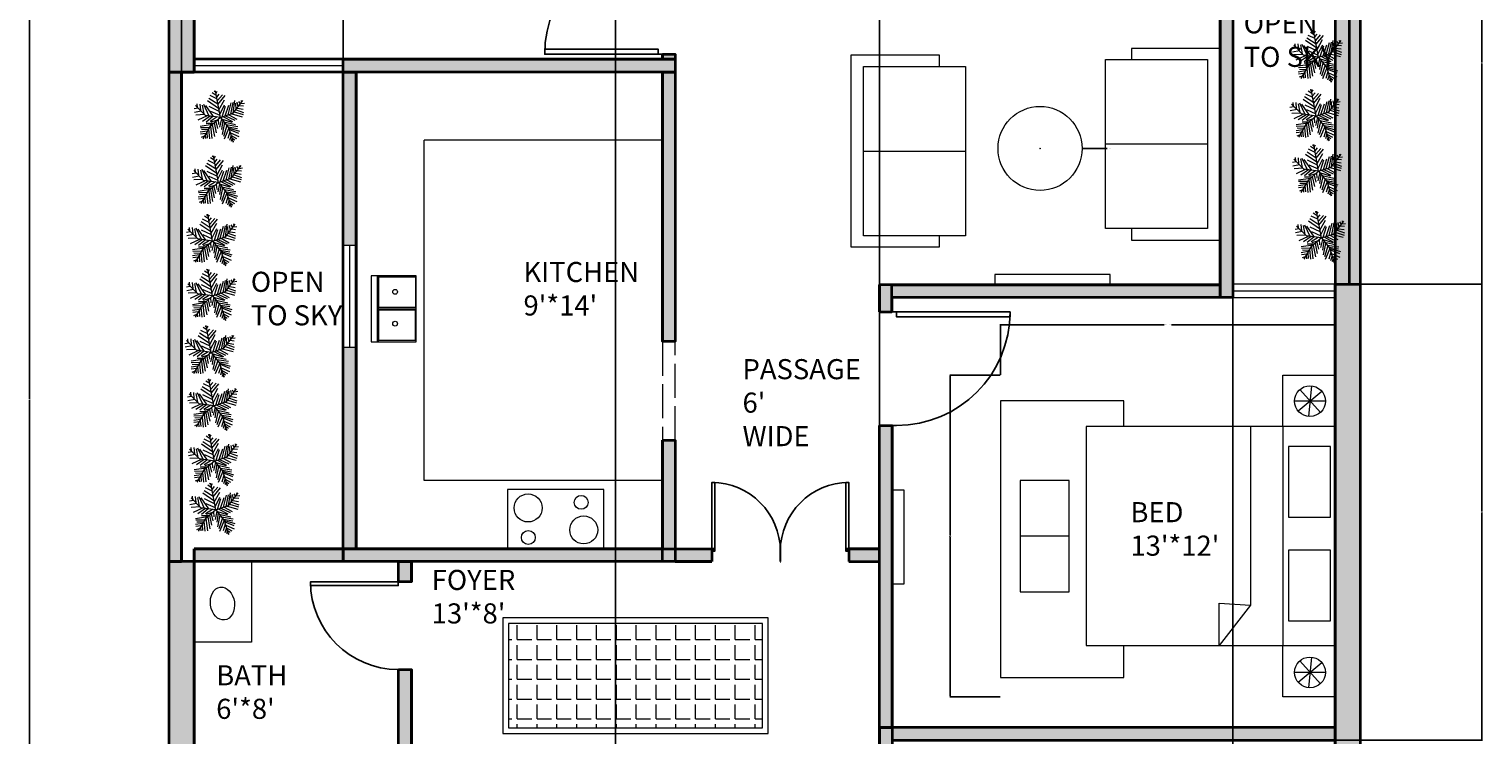
# Model space of a CAD drawing. Units: inches. Extents: x 2119 to 2631, y 2040 to 2935.
# Tile 2 of 3: x 2119 to 2631, y 2369 to 2618. Entities that reach past the tile are written whole.
import ezdxf

# ---------------------------------------------------------------- set-up
doc = ezdxf.new("R2010")
doc.units = ezdxf.units.IN
doc.linetypes.add('ACAD_ISO02W100', pattern=[15, 12, -3])
for name, color, linetype, lineweight in [('A-ANNO-DIMS', 2, 'Continuous', 18), ('A-AREA-IDEN', 7, 'Continuous', 18), ('A-EQPM', 8, 'Continuous', 18), ('A-FLOR-CASE', 33, 'Continuous', 18), ('A-FLOR-FIXT', 9, 'Continuous', 18), ('A-FLOR-PATT', 9, 'Continuous', 13), ('A-WALL-OVHD', 180, 'ACAD_ISO02W100', 18), ('A-WALL-PATT', 252, 'Continuous', 13), ('C-PROP', 7, 'Continuous', 35), ('DOOR', 50, 'Continuous', 25), ('FURNITURE', 220, 'Continuous', 18), ('GRASS', 70, 'Continuous', 13), ('WALL', 180, 'Continuous', 35), ('WINDOW', 130, 'Continuous', 18)]:
    doc.layers.add(name, color=color, linetype=linetype, lineweight=lineweight)
doc.styles.get("Standard").update_dxf_attribs({"font": 'arial.ttf'})
doc.dimstyles.get("Standard").update_dxf_attribs({"dimtxt": 0.18, "dimasz": 0.18, "dimexe": 0.18, "dimexo": 0.0625, "dimgap": 0.09, "dimtad": 0, "dimtih": 1, "dimtoh": 1, "dimdec": 4, "dimzin": 0, "dimdsep": 46, "dimtxsty": 'Standard', "dimcen": 0.09, "dimadec": 0, "dimazin": 0, "dimtfac": 1, "dimtdec": 4, "dimtofl": 0, "dimtmove": 0, "dimatfit": 3, "dimfxl": 1, "dimtolj": 1, "dimtzin": 0, "dimarcsym": 0})

# ---------------------------------------------------------------- blocks, each defined once
blk = doc.blocks.new('*U2')
for p, q in [((0, 0), (0, -6)), ((40, 0), (40, -6))]:
    blk.add_line(p, q)
blk.add_lwpolyline([(0, 0), (0, 40), (1.75, 40), (1.75, 0)], close=True)
blk.add_arc((0, 0), 40, 0, 90)
blk = doc.blocks.new('*U6')
for p, q in [((-3.665, 19.273), (-27.574, 35.527)), ((-5.114, 28.097), (-24.676, 40.636)), ((-7.288, 39.707), (-21.778, 46.673)), ((-8.737, 47.138), (-17.069, 52.711)), ((-10.186, 53.64), (-13.084, 55.962)), ((0, 0), (-10.5, 57)), ((-9.099, 51.782), (-6.563, 55.962)), ((-7.65, 43.423), (-2.578, 49.46)), ((-5.839, 35.992), (4.667, 48.067)), ((-5.114, 27.632), (10.463, 46.673)), ((-2.941, 16.486), (8.652, 37.85)), ((16.259, 5.805), (23.142, 31.348)), ((22.055, 7.198), (27.489, 32.277)), ((27, 9), (48, 36)), ((27.127, 9.056), (31.112, 35.992)), ((35.096, 32.741), (37.27, 22.524)), ((38.719, 34.134), (41.979, 28.561)), ((44.153, 36.456), (45.239, 32.741)), ((-47.498, 19.737), (-55.83, 18.344)), ((-40.615, 13.7), (-55.105, 10.913)), ((-31.5, 4.5), (-52.5, 25.5)), ((-33.37, 6.269), (-52.207, 5.34)), ((-48.585, 21.131), (-49.309, 29.026)), ((-28.299, 3.483), (-47.86, -5.805)), ((-43.513, 28.561), (-42.427, 15.558)), ((-38.442, 26.239), (-34.819, 7.663)), ((-21.416, 3.018), (-38.079, -8.128)), ((-35.544, 28.097), (-24.314, 3.947)), ((0, 0), (-31.5, 4.5)), ((-14.533, 2.09), (-30.834, 25.31)), ((-15.982, 2.09), (-30.11, -9.521)), ((-24.314, 23.917), (-2.941, 13.7)), ((0, 0), (-22.5, -19.5)), ((-6.563, 1.161), (-21.416, -8.128)), ((-20.691, 13.7), (-1.129, 4.876)), ((-1.129, 6.734), (9.014, 26.704)), ((0, 0), (27, 9)), ((0, 0), (18, -22.5)), ((3.942, 1.625), (11.187, 24.381)), ((6.478, 1.625), (26.04, -8.592)), ((10.101, 3.483), (17.708, 26.239)), ((11.187, 3.483), (30.749, -5.805)), ((18.07, 5.805), (35.096, -3.483)), ((24.229, 7.663), (46.688, 1.625)), ((29.662, 12.307), (48.137, 6.269)), ((31.836, 30.883), (32.561, 16.486)), ((33.285, 16.486), (48.862, 10.913)), ((36.183, 19.737), (48.137, 17.88)), ((40.53, 25.775), (48.862, 24.846)), ((43.791, 29.954), (51.036, 30.883)), ((-17.431, -15.094), (-42.789, -18.809)), ((-28.299, -29.026), (-42.789, -31.348)), ((-24.314, -21.596), (-42.427, -22.06)), ((-26.849, -26.24), (-40.253, -25.775)), ((-22.5, -19.5), (-37.5, -45)), ((-15.257, -12.772), (-30.11, -12.772)), ((-29.023, -30.884), (-27.936, -43.887)), ((-25.038, -23.918), (-22.865, -45.281)), ((-20.691, -18.345), (-17.793, -44.352)), ((-6.563, -5.805), (-19.967, -9.985)), ((-17.069, -15.094), (-12.721, -40.172)), ((-13.446, -11.378), (-8.737, -32.741)), ((-9.461, -8.592), (-6.201, -23.453)), ((-4.752, -3.483), (-3.665, -14.629)), ((2.493, -3.019), (-1.491, -20.202)), ((1.769, -2.555), (24.229, -9.521)), ((5.029, -6.27), (2.131, -25.775)), ((9.014, -11.378), (3.58, -35.992)), ((14.085, -16.951), (6.478, -40.172)), ((7.565, -9.056), (32.198, -14.629)), ((18.07, -22.524), (8.289, -45.745)), ((12.274, -15.094), (36.907, -18.809)), ((20.244, -30.419), (15.897, -44.816)), ((16.259, -19.738), (36.183, -22.989)), ((18, -22.5), (27, -52.5)), ((18.433, -22.524), (40.53, -29.026)), ((19.157, -25.311), (38.719, -33.206)), ((-30.834, -34.135), (-42.427, -35.528)), ((-34.457, -39.708), (-40.978, -42.494)), ((-32.646, -36.921), (-31.921, -44.352)), ((22.78, -37.85), (19.519, -48.532)), ((21.331, -32.741), (39.081, -40.636)), ((22.78, -38.314), (34.372, -44.816)), ((24.591, -45.745), (23.142, -50.854)), ((24.591, -43.423), (30.749, -47.603)), ((26.764, -49.925), (28.213, -50.854))]:
    blk.add_line(p, q)
blk = doc.blocks.new('BED-DOUBLE-SUITE')
for p, q in [((-13.02, 5.47), (-4.66, 12.4)), ((-12.38, 13.04), (-5.14, 4.94)), ((-9.21, 3.5), (-8.22, 14.32)), ((-74.36, 9.08), (-117.92, 9.08)), ((-117.92, 9.08), (-117.92, -88.45)), ((-74.36, 0), (-74.36, 9.08)), ((-14.26, 9.02), (-3.4, 8.97)), ((-29.81, 0), (-29.81, -62.95)), ((-18.41, 0), (-18.41, -77.17)), ((-93.69, -38.69), (-110.95, -38.69)), ((-40.83, -77.17), (-40.83, -62.28)), ((-40.83, -62.28), (-29.81, -62.95)), ((-29.81, -62.95), (-40.83, -77.17)), ((-74.36, -88.45), (-74.36, -77.17)), ((-9.21, -92.12), (-8.22, -81.31)), ((-14.26, -86.6), (-3.4, -86.65)), ((-13.02, -90.15), (-4.66, -83.22)), ((-12.38, -82.59), (-5.14, -90.68)), ((-117.92, -88.45), (-74.36, -88.45))]:
    blk.add_line(p, q)
for points in [[(0, 0), (-18.39, 0), (-18.39, 18.13), (0, 18.13)], [(0, 0), (-87.71, 0), (-87.71, -77.17), (0, -77.17)], [(-1.58, -7.03), (-16.39, -7.03), (-16.39, -31.92), (-1.58, -31.92)], [(-93.69, -19.1), (-110.95, -19.1), (-110.95, -58.28), (-93.69, -58.28)], [(-1.58, -43.58), (-16.39, -43.58), (-16.39, -68.47), (-1.58, -68.47)], [(0, -95.3), (-18.39, -95.3), (-18.39, -77.17), (0, -77.17)]]:
    blk.add_lwpolyline(points, close=True)
for centre in [(-8.83, 8.92), (-8.83, -86.7)]:
    blk.add_circle(centre, 5.43)
blk = doc.blocks.new('SOFA-2-SEAT')
for p, q in [((-9.19, 63.72), (-40.39, 63.72)), ((-40.39, 63.72), (-40.39, -3.87)), ((-9.19, 59.66), (-9.19, 63.72)), ((-35.92, 29.83), (0, 29.83)), ((-9.19, -3.87), (-9.19, 0)), ((-40.39, -3.87), (-9.19, -3.87))]:
    blk.add_line(p, q)
blk.add_lwpolyline([(0, 0), (-35.92, 0), (-35.92, 59.66), (0, 59.66)], close=True)
blk = doc.blocks.new('BASIN-VANITY')
blk.add_lwpolyline([(0, 0), (-20.15, 0), (-20.15, 28.46), (0, 28.46)], close=True)
blk.add_ellipse((-10.21, 13.63), major_axis=(0.77, -5.8), ratio=0.722636)
blk = doc.blocks.new('*D12')
at = {"layer": 'A-ANNO-DIMS', "color": 0, "lineweight": -2, "transparency": 16777216}
for p, q in [((2461.34, 2496.18), (2461.34, 2513.99)), ((2461.52, 2513.81), (2519, 2513.81)), ((2579.07, 2513.81), (2521.59, 2513.81)), ((2579.25, 2496.18), (2579.25, 2513.99))]:
    blk.add_line(p, q, dxfattribs=at)
at = {"layer": 'A-ANNO-DIMS', "color": 0, "lineweight": 100, "transparency": 16777216}
for points in [[(2461.52, 2513.84), (2461.52, 2513.78), (2461.34, 2513.81)], [(2579.07, 2513.84), (2579.07, 2513.78), (2579.25, 2513.81)]]:
    blk.add_solid(points, dxfattribs=at)
at = {"layer": 'Defpoints', "color": 0, "lineweight": 100, "transparency": 16777216}
for p in [(2579.25, 2513.81), (2461.34, 2496.12), (2579.25, 2496.12)]:
    blk.add_point(p, dxfattribs=at)
at = {"layer": 'A-ANNO-DIMS', "color": 0, "transparency": 16777216, "insert": (2520.3, 2513.81), "char_height": 0.18, "attachment_point": 5}
blk.add_mtext('\\A1;BED SUITE 118 TYP.', dxfattribs=at)
blk = doc.blocks.new('*D13')
at = {"layer": 'A-ANNO-DIMS', "color": 0, "lineweight": -2, "transparency": 16777216}
for p, q in [((2461.28, 2496.12), (2443.47, 2496.12)), ((2443.65, 2495.94), (2443.65, 2439.59)), ((2443.65, 2382.87), (2443.65, 2439.22)), ((2461.28, 2382.69), (2443.47, 2382.69))]:
    blk.add_line(p, q, dxfattribs=at)
at = {"layer": 'A-ANNO-DIMS', "color": 0, "lineweight": 100, "transparency": 16777216}
for points in [[(2443.62, 2495.94), (2443.68, 2495.94), (2443.65, 2496.12)], [(2443.62, 2382.87), (2443.68, 2382.87), (2443.65, 2382.69)]]:
    blk.add_solid(points, dxfattribs=at)
at = {"layer": 'Defpoints', "color": 0, "lineweight": 100, "transparency": 16777216}
for p in [(2443.65, 2496.12), (2461.34, 2496.12), (2461.34, 2382.69)]:
    blk.add_point(p, dxfattribs=at)
at = {"layer": 'A-ANNO-DIMS', "color": 0, "transparency": 16777216, "insert": (2443.65, 2439.4), "char_height": 0.18, "attachment_point": 5}
blk.add_mtext('\\A1;113 TYP.', dxfattribs=at)
blk = doc.blocks.new('*D19')
at = {"layer": 'A-ANNO-DIMS', "color": 0, "lineweight": -2, "transparency": 16777216}
for p, q in [((2168.19, 2877.4), (2119.07, 2877.4)), ((2119.25, 2877.22), (2119.25, 2487.58)), ((2119.25, 2097.58), (2119.25, 2487.22)), ((2168.19, 2097.4), (2119.07, 2097.4))]:
    blk.add_line(p, q, dxfattribs=at)
at = {"layer": 'A-ANNO-DIMS', "color": 0, "lineweight": 100, "transparency": 16777216}
for points in [[(2119.22, 2877.22), (2119.28, 2877.22), (2119.25, 2877.4)], [(2119.22, 2097.58), (2119.28, 2097.58), (2119.25, 2097.4)]]:
    blk.add_solid(points, dxfattribs=at)
at = {"layer": 'Defpoints', "color": 0, "lineweight": 100, "transparency": 16777216}
for p in [(2119.25, 2877.4), (2168.25, 2877.4), (2168.25, 2097.4)]:
    blk.add_point(p, dxfattribs=at)
at = {"layer": 'A-ANNO-DIMS', "color": 0, "transparency": 16777216, "insert": (2119.25, 2487.4), "char_height": 0.18, "attachment_point": 5}
blk.add_mtext('\\A1;780', dxfattribs=at)
blk = doc.blocks.new('*D21')
at = {"layer": 'A-ANNO-DIMS', "color": 0, "lineweight": -2, "transparency": 16777216}
for p, q in [((2325.75, 2175.46), (2325.75, 2934.76)), ((2325.93, 2934.58), (2372.04, 2934.58)), ((2418.57, 2934.58), (2372.47, 2934.58)), ((2418.75, 2175.46), (2418.75, 2934.76))]:
    blk.add_line(p, q, dxfattribs=at)
at = {"layer": 'A-ANNO-DIMS', "color": 0, "lineweight": 100, "transparency": 16777216}
for points in [[(2325.93, 2934.61), (2325.93, 2934.55), (2325.75, 2934.58)], [(2418.57, 2934.61), (2418.57, 2934.55), (2418.75, 2934.58)]]:
    blk.add_solid(points, dxfattribs=at)
at = {"layer": 'Defpoints', "color": 0, "lineweight": 100, "transparency": 16777216}
for p in [(2418.75, 2934.58), (2325.75, 2175.4), (2418.75, 2175.4)]:
    blk.add_point(p, dxfattribs=at)
at = {"layer": 'A-ANNO-DIMS', "color": 0, "transparency": 16777216, "insert": (2372.25, 2934.58), "char_height": 0.18, "attachment_point": 5}
blk.add_mtext('\\A1;93', dxfattribs=at)
blk = doc.blocks.new('*D24')
at = {"layer": 'A-ANNO-DIMS', "color": 0, "lineweight": -2, "transparency": 16777216}
for p, q in [((2588.32, 2528.16), (2631.18, 2528.16)), ((2631, 2527.98), (2631, 2447.96)), ((2631, 2367.58), (2631, 2447.6)), ((2579.32, 2367.4), (2631.18, 2367.4))]:
    blk.add_line(p, q, dxfattribs=at)
at = {"layer": 'A-ANNO-DIMS', "color": 0, "lineweight": 100, "transparency": 16777216}
for points in [[(2630.97, 2527.98), (2631.03, 2527.98), (2631, 2528.16)], [(2630.97, 2367.58), (2631.03, 2367.58), (2631, 2367.4)]]:
    blk.add_solid(points, dxfattribs=at)
at = {"layer": 'Defpoints', "color": 0, "lineweight": 100, "transparency": 16777216}
for p in [(2588.25, 2528.16), (2631, 2528.16), (2579.25, 2367.4)]:
    blk.add_point(p, dxfattribs=at)
at = {"layer": 'A-ANNO-DIMS', "color": 0, "transparency": 16777216, "insert": (2631, 2447.78), "char_height": 0.18, "attachment_point": 5}
blk.add_mtext('\\A1;160.76', dxfattribs=at)
blk = doc.blocks.new('*D25')
at = {"layer": 'A-ANNO-DIMS', "color": 0, "lineweight": -2, "transparency": 16777216}
for p, q in [((2588.32, 2683.9), (2631.18, 2683.9)), ((2631, 2683.72), (2631, 2606.21)), ((2631, 2528.34), (2631, 2605.85)), ((2588.32, 2528.16), (2631.18, 2528.16))]:
    blk.add_line(p, q, dxfattribs=at)
at = {"layer": 'A-ANNO-DIMS', "color": 0, "lineweight": 100, "transparency": 16777216}
for points in [[(2630.97, 2683.72), (2631.03, 2683.72), (2631, 2683.9)], [(2630.97, 2528.34), (2631.03, 2528.34), (2631, 2528.16)]]:
    blk.add_solid(points, dxfattribs=at)
at = {"layer": 'Defpoints', "color": 0, "lineweight": 100, "transparency": 16777216}
for p in [(2588.25, 2683.9), (2631, 2683.9), (2588.25, 2528.16)]:
    blk.add_point(p, dxfattribs=at)
at = {"layer": 'A-ANNO-DIMS', "color": 0, "transparency": 16777216, "insert": (2631, 2606.03), "char_height": 0.18, "attachment_point": 5}
blk.add_mtext('\\A1;155.74', dxfattribs=at)
blk = doc.blocks.new('*D30')
at = {"layer": 'A-ANNO-DIMS', "color": 0, "lineweight": -2, "transparency": 16777216}
for p, q in [((2172.75, 2602.96), (2172.75, 2645.83)), ((2172.93, 2645.65), (2201.04, 2645.65)), ((2229.57, 2645.65), (2201.47, 2645.65)), ((2229.75, 2602.96), (2229.75, 2645.83))]:
    blk.add_line(p, q, dxfattribs=at)
at = {"layer": 'A-ANNO-DIMS', "color": 0, "lineweight": 100, "transparency": 16777216}
for points in [[(2172.93, 2645.68), (2172.93, 2645.62), (2172.75, 2645.65)], [(2229.57, 2645.68), (2229.57, 2645.62), (2229.75, 2645.65)]]:
    blk.add_solid(points, dxfattribs=at)
at = {"layer": 'Defpoints', "color": 0, "lineweight": 100, "transparency": 16777216}
for p in [(2229.75, 2645.65), (2172.75, 2602.9), (2229.75, 2602.9)]:
    blk.add_point(p, dxfattribs=at)
at = {"layer": 'A-ANNO-DIMS', "color": 0, "transparency": 16777216, "insert": (2201.25, 2645.65), "char_height": 0.18, "attachment_point": 5}
blk.add_mtext('\\A1;57', dxfattribs=at)
blk = doc.blocks.new('*D31')
at = {"layer": 'A-ANNO-DIMS', "color": 0, "lineweight": -2, "transparency": 16777216}
for p, q in [((2543.25, 2683.84), (2543.25, 2054.47)), ((2579.25, 2683.84), (2579.25, 2054.47)), ((2543.43, 2054.65), (2561.04, 2054.65)), ((2579.07, 2054.65), (2561.47, 2054.65))]:
    blk.add_line(p, q, dxfattribs=at)
at = {"layer": 'A-ANNO-DIMS', "color": 0, "lineweight": 100, "transparency": 16777216}
for points in [[(2543.43, 2054.68), (2543.43, 2054.62), (2543.25, 2054.65)], [(2579.07, 2054.68), (2579.07, 2054.62), (2579.25, 2054.65)]]:
    blk.add_solid(points, dxfattribs=at)
at = {"layer": 'Defpoints', "color": 0, "lineweight": 100, "transparency": 16777216}
for p in [(2543.25, 2683.9), (2579.25, 2683.9), (2579.25, 2054.65)]:
    blk.add_point(p, dxfattribs=at)
at = {"layer": 'A-ANNO-DIMS', "color": 0, "transparency": 16777216, "insert": (2561.25, 2054.65), "char_height": 0.18, "attachment_point": 5}
blk.add_mtext('\\A1;36', dxfattribs=at)
blk = doc.blocks.new('*D33')
at = {"layer": 'A-ANNO-DIMS', "color": 0, "lineweight": -2, "transparency": 16777216}
for p, q in [((2475.21, 2575.97), (2475.39, 2575.97)), ((2475.3, 2575.88), (2475.3, 2576.06)), ((2498.99, 2575.97), (2490.29, 2575.97))]:
    blk.add_line(p, q, dxfattribs=at)
at = {"layer": 'A-ANNO-DIMS', "color": 0, "lineweight": 100, "transparency": 16777216}
blk.add_solid([(2490.29, 2576), (2490.29, 2575.94), (2490.11, 2575.97)], dxfattribs=at)
at = {"layer": 'Defpoints', "color": 0, "lineweight": 100, "transparency": 16777216}
for p in [(2460.5, 2575.97), (2490.11, 2575.97)]:
    blk.add_point(p, dxfattribs=at)
at = {"layer": 'A-ANNO-DIMS', "color": 0, "transparency": 16777216, "insert": (2499.55, 2575.97), "char_height": 0.18, "attachment_point": 5}
blk.add_mtext('\\A1;∅29.605', dxfattribs=at)

msp = doc.modelspace()

# ---------------------------------------------------------------- hatches: boundary and pattern name
at = {"layer": 'A-FLOR-PATT'}
h = msp.add_hatch(dxfattribs=at)
h.set_pattern_fill('ANGLE', color=256)
h.set_pattern_definition([(0, (0, 0), (0, 6.985), [5.08, -1.905]), (90, (0, 0), (-6.985, 4e-16), [5.08, -1.905])])
h.paths.add_polyline_path([(2377.4508, 2408.5471), (2288.0046, 2408.5471), (2288.0046, 2371.7403), (2377.4508, 2371.7403)])
at = {"layer": 'A-WALL-PATT'}
h = msp.add_hatch(color=256, dxfattribs=at)
h.dxf.hatch_style = 1
h.paths.add_polyline_path([(2177.2549, 2868.3983), (2168.2549, 2868.3983), (2168.2549, 2602.8983), (2177.2549, 2602.8983)])
h.paths.add_polyline_path([(2588.2549, 2877.3983), (2579.2549, 2877.3983), (2579.2549, 2868.6805), (2588.2549, 2868.6805)])
h.paths.add_polyline_path([(2579.2549, 2877.3983), (2168.2549, 2877.3983), (2168.2549, 2868.6805), (2579.2549, 2868.6805)])
h.paths.add_polyline_path([(2588.2549, 2868.6805), (2579.2549, 2868.6805), (2579.2549, 2166.3983), (2588.2549, 2166.3983)])
h = msp.add_hatch(color=256, dxfattribs=at)
h.dxf.hatch_style = 1
h.paths.add_polyline_path([(2543.2549, 2683.8983), (2538.7549, 2683.8983), (2538.7549, 2523.3983), (2543.2549, 2523.3983)])
h = msp.add_hatch(color=256, dxfattribs=at)
h.dxf.hatch_style = 1
h.paths.add_polyline_path([(2177.2549, 2430.3983), (2168.2549, 2430.3983), (2168.2549, 2097.3983), (2177.2549, 2097.3983)])
h.paths.add_polyline_path([(2172.7549, 2602.8983), (2168.2549, 2602.8983), (2168.2549, 2430.3983), (2172.7549, 2430.3983)])
h.paths.add_polyline_path([(2229.7549, 2434.8983), (2177.2549, 2434.8983), (2177.2549, 2430.3983), (2229.7549, 2430.3983)])
h.paths.add_polyline_path([(2342.2549, 2434.8983), (2229.7549, 2434.8983), (2229.7549, 2430.3983), (2342.2549, 2430.3983)])
h.paths.add_polyline_path([(2359.6188, 2434.8983), (2346.7549, 2434.8983), (2346.7549, 2430.3983), (2359.6188, 2430.3983)])
h.paths.add_polyline_path([(2346.7549, 2434.8983), (2342.2549, 2434.8983), (2342.2549, 2430.3983), (2346.7549, 2430.3983)])
h.paths.add_polyline_path([(2346.7549, 2602.8983), (2342.2549, 2602.8983), (2342.2549, 2507.872), (2346.7549, 2507.872)])
h.paths.add_polyline_path([(2346.7549, 2609.1862), (2342.2549, 2609.1862), (2342.2549, 2607.3983), (2346.7549, 2607.3983)])
h.paths.add_polyline_path([(2346.7549, 2607.3983), (2342.2549, 2607.3983), (2229.7549, 2607.3983), (2229.7549, 2602.8983), (2346.7549, 2602.8983)])
h = msp.add_hatch(color=256, dxfattribs=at)
h.dxf.hatch_style = 1
h.paths.add_polyline_path([(2538.7549, 2527.8983), (2423.1333, 2527.8983), (2423.1333, 2523.3983), (2538.7549, 2523.3983)])
h.paths.add_polyline_path([(2234.2549, 2602.8983), (2229.7549, 2602.8983), (2229.7549, 2541.8001), (2234.2549, 2541.8001)])
h.paths.add_polyline_path([(2253.7549, 2392.3266), (2249.2549, 2392.3266), (2249.2549, 2334.3983), (2253.7549, 2334.3983)])
h.paths.add_polyline_path([(2249.2549, 2334.3983), (2211.4668, 2334.3983), (2211.4668, 2329.8983), (2249.2549, 2329.8983)])
h.paths.add_polyline_path([(2258.3247, 2334.3983), (2253.7549, 2334.3983), (2253.7549, 2329.8983), (2258.3247, 2329.8983)])
h.paths.add_polyline_path([(2253.7549, 2334.3983), (2249.2549, 2334.3983), (2249.2549, 2329.8983), (2253.7549, 2329.8983)])
h.paths.add_polyline_path([(2187.4668, 2334.3983), (2177.2549, 2334.3983), (2177.2549, 2329.8983), (2187.4668, 2329.8983)])
h.paths.add_polyline_path([(2253.7549, 2430.3983), (2249.2549, 2430.3983), (2249.2549, 2423.2235), (2253.7549, 2423.2235)])
h.paths.add_polyline_path([(2579.2549, 2371.8983), (2423.2549, 2371.8983), (2423.2549, 2367.3983), (2579.2549, 2367.3983)])
h.paths.add_polyline_path([(2423.2549, 2371.8983), (2418.7549, 2371.8983), (2418.7549, 2338.9216), (2423.2549, 2338.9216)])
h = msp.add_hatch(color=256, dxfattribs=at)
h.dxf.hatch_style = 1
h.paths.add_polyline_path([(2423.2549, 2478.3647), (2418.7549, 2478.3647), (2418.7549, 2371.8983), (2423.2549, 2371.8983)])
h.paths.add_polyline_path([(2418.7549, 2434.8983), (2407.9569, 2434.8983), (2407.9569, 2430.3983), (2418.7549, 2430.3983)])
h.paths.add_polyline_path([(2346.7549, 2473.1113), (2342.2549, 2473.1113), (2342.2549, 2434.8983), (2346.7549, 2434.8983)])
h.paths.add_polyline_path([(2234.2549, 2505.8001), (2229.7549, 2505.8001), (2229.7549, 2434.8983), (2234.2549, 2434.8983)])
h.paths.add_polyline_path([(2423.1333, 2527.8983), (2418.7549, 2527.8983), (2418.7549, 2518.3647), (2423.1333, 2518.3647)])

# ---------------------------------------------------------------- linework, layer by layer
at = {"layer": 'A-EQPM'}
for points in [[(2459.3947, 2527.8983), (2499.9711, 2527.8983), (2499.9711, 2531.5047), (2459.3947, 2531.5047)], [(2287.6055, 2434.8983), (2321.5347, 2434.8983), (2321.5347, 2455.7091), (2287.6055, 2455.7091)], [(2423.2549, 2422.4993), (2427.4168, 2422.4993), (2427.4168, 2455.5332), (2423.2549, 2455.5332)]]:
    msp.add_lwpolyline(points, close=True, dxfattribs=at)
for centre, radius in [((2294.9156, 2449.2629), 4.9368), ((2313.6117, 2451.2264), 2.4399), ((2314.5101, 2441.5212), 4.9368), ((2294.9718, 2438.8284), 2.4399)]:
    msp.add_circle(centre, radius, dxfattribs=at)
at = {"layer": 'A-FLOR-CASE'}
for p, q in [((2342.2549, 2602.8983), (2342.2549, 2578.8983)), ((2258.2549, 2458.8983), (2258.2549, 2578.8983)), ((2342.2549, 2578.8983), (2258.2549, 2578.8983)), ((2342.2549, 2458.8983), (2258.2549, 2458.8983)), ((2342.2549, 2434.8983), (2342.2549, 2458.8983)), ((2234.2549, 2434.8983), (2258.2549, 2434.8983))]:
    msp.add_line(p, q, dxfattribs=at)
at = {"layer": 'A-FLOR-FIXT'}
for p, q in [((2241.6697, 2531.0764), (2241.6697, 2507.8088)), ((2242.0071, 2531.0764), (2242.0071, 2507.8088)), ((2242.0071, 2519.4426), (2255.4928, 2519.4426))]:
    msp.add_line(p, q, dxfattribs=at)
for points in [[(2239.5375, 2507.8088), (2255.4928, 2507.8088), (2255.4928, 2531.0764), (2239.5375, 2531.0764)], [(2242.3032, 2530.7064), (2255.2262, 2530.7064), (2255.2262, 2519.8696), (2242.3032, 2519.8696)], [(2242.3384, 2519.0604), (2255.113, 2519.0604), (2255.113, 2508.2464), (2242.3384, 2508.2464)]]:
    msp.add_lwpolyline(points, close=True, dxfattribs=at)
for centre in [(2248.0276, 2525.4273), (2248.0276, 2514.2222)]:
    msp.add_circle(centre, 0.8453, dxfattribs=at)
at = {"layer": 'A-WALL-OVHD'}
msp.add_lwpolyline([(2342.2549, 2473.1113), (2346.7549, 2473.1113), (2346.7549, 2507.872), (2342.2549, 2507.872)], close=True, dxfattribs=at)
at = {"layer": 'C-PROP'}
msp.add_lwpolyline([(2168.2549, 2097.3983), (2588.2549, 2097.3983), (2588.2549, 2877.3983), (2168.2549, 2877.3983)], close=True, dxfattribs=at)
at = {"layer": 'FURNITURE'}
for points in [[(2286.0046, 2369.7403), (2379.4508, 2369.7403), (2379.4508, 2410.5471), (2286.0046, 2410.5471)], [(2288.0046, 2371.7403), (2377.4508, 2371.7403), (2377.4508, 2408.5471), (2288.0046, 2408.5471)]]:
    msp.add_lwpolyline(points, close=True, dxfattribs=at)
msp.add_circle((2475.3026, 2575.9729), 14.8026, dxfattribs=at)
at = {"layer": 'WALL'}
for p, q in [((2538.7549, 2683.8983), (2538.7549, 2527.8983)), ((2543.2549, 2683.8983), (2543.2549, 2523.3983)), ((2584.2794, 2683.8983), (2584.2794, 2528.1615)), ((2342.2549, 2609.1862), (2342.2549, 2607.3983)), ((2346.7549, 2609.1862), (2346.7549, 2602.8983)), ((2177.2549, 2602.8983), (2168.2549, 2602.8983)), ((2172.7549, 2602.8983), (2172.7549, 2430.3983)), ((2186.2549, 2607.3983), (2177.2549, 2607.3983)), ((2186.2549, 2602.8983), (2177.2549, 2602.8983)), ((2342.2549, 2607.3983), (2186.2549, 2607.3983)), ((2346.7549, 2602.8983), (2186.2549, 2602.8983)), ((2229.7549, 2430.3983), (2229.7549, 2602.8983)), ((2234.2549, 2434.8983), (2234.2549, 2602.8983)), ((2342.2549, 2602.8983), (2342.2549, 2507.872)), ((2346.7549, 2602.8983), (2346.7549, 2507.872)), ((2538.7549, 2527.8983), (2418.7549, 2527.8983)), ((2418.7549, 2518.3647), (2418.7549, 2527.8983)), ((2579.2549, 2528.1615), (2588.2549, 2528.1615)), ((2543.2549, 2523.3983), (2423.2549, 2523.3983)), ((2423.2549, 2518.3647), (2423.2549, 2523.3983)), ((2579.2549, 2500.8813), (2579.2549, 2373.4565)), ((2418.7549, 2434.8983), (2418.7549, 2478.3647)), ((2423.2549, 2371.8983), (2423.2549, 2478.3647)), ((2342.2549, 2473.1113), (2342.2549, 2434.8983)), ((2346.7549, 2473.1113), (2346.7549, 2434.8983)), ((2229.7549, 2434.8983), (2177.2549, 2434.8983)), ((2342.2549, 2434.8983), (2234.2549, 2434.8983)), ((2346.7549, 2434.8983), (2360.6767, 2434.8983)), ((2383.7821, 2434.8983), (2383.7936, 2434.8983)), ((2406.899, 2434.8983), (2418.7549, 2434.8983)), ((2177.2549, 2430.3983), (2168.2549, 2430.3983)), ((2229.7549, 2430.3983), (2177.2549, 2430.3983)), ((2177.2549, 2430.3983), (2177.2549, 2334.3983)), ((2346.7549, 2430.3983), (2229.7549, 2430.3983)), ((2249.2549, 2423.2235), (2249.2549, 2430.3983)), ((2253.7549, 2423.2235), (2253.7549, 2430.3983)), ((2346.7549, 2430.3983), (2359.6188, 2430.3983)), ((2383.7779, 2430.3983), (2383.7979, 2430.3983)), ((2407.9569, 2430.3983), (2418.7549, 2430.3983)), ((2418.7549, 2371.8983), (2418.7549, 2430.3983)), ((2249.2549, 2334.3983), (2249.2549, 2392.3266)), ((2253.7549, 2329.8983), (2253.7549, 2392.3266)), ((2579.2549, 2371.8983), (2418.7549, 2371.8983)), ((2418.7549, 2371.8983), (2418.7549, 2338.9216))]:
    msp.add_line(p, q, dxfattribs=at)
for points in [[(2588.2549, 2877.3983), (2579.2549, 2877.3983), (2579.2549, 2166.3983), (2588.2549, 2166.3983)], [(2168.2549, 2602.8983), (2177.2549, 2602.8983), (2177.2549, 2868.3983), (2168.2549, 2868.3983)], [(2538.7549, 2683.8983), (2543.2549, 2683.8983), (2543.2549, 2523.3983), (2538.7549, 2523.3983)], [(2342.2549, 2609.1862), (2346.7549, 2609.1862), (2346.7549, 2607.3983), (2342.2549, 2607.3983)], [(2168.2549, 2430.3983), (2172.7549, 2430.3983), (2172.7549, 2602.8983), (2168.2549, 2602.8983)], [(2229.7549, 2607.3983), (2346.7549, 2607.3983), (2346.7549, 2602.8983), (2229.7549, 2602.8983)], [(2229.7549, 2602.8983), (2234.2549, 2602.8983), (2234.2549, 2434.8983), (2229.7549, 2434.8983)], [(2342.2549, 2602.8983), (2346.7549, 2602.8983), (2346.7549, 2507.872), (2342.2549, 2507.872)], [(2418.7549, 2518.3647), (2423.1333, 2518.3647), (2423.1333, 2527.8983), (2418.7549, 2527.8983)], [(2423.1333, 2527.8983), (2538.7549, 2527.8983), (2538.7549, 2523.3983), (2423.1333, 2523.3983)], [(2418.7549, 2478.3647), (2423.2549, 2478.3647), (2423.2549, 2371.8983), (2418.7549, 2371.8983)], [(2342.2549, 2473.1113), (2346.7549, 2473.1113), (2346.7549, 2430.3983), (2342.2549, 2430.3983)], [(2177.2549, 2434.8983), (2229.7549, 2434.8983), (2229.7549, 2430.3983), (2177.2549, 2430.3983)], [(2359.6188, 2430.3983), (2229.7549, 2430.3983), (2229.7549, 2434.8983), (2359.6188, 2434.8983)], [(2407.9569, 2430.3983), (2418.7549, 2430.3983), (2418.7549, 2434.8983), (2407.9569, 2434.8983)], [(2168.2549, 2097.3983), (2177.2549, 2097.3983), (2177.2549, 2430.3983), (2168.2549, 2430.3983)], [(2249.2549, 2430.3983), (2253.7549, 2430.3983), (2253.7549, 2423.2235), (2249.2549, 2423.2235)], [(2249.2549, 2392.3266), (2253.7549, 2392.3266), (2253.7549, 2329.8983), (2249.2549, 2329.8983)], [(2418.7549, 2371.8983), (2423.2549, 2371.8983), (2423.2549, 2338.9216), (2418.7549, 2338.9216)], [(2579.2549, 2371.8983), (2423.2549, 2371.8983), (2423.2549, 2367.3983), (2579.2549, 2367.3983)]]:
    msp.add_lwpolyline(points, close=True, dxfattribs=at)
for points in [[(2342.2549, 2868.3983), (2177.2549, 2868.3983), (2177.2549, 2602.8983)], [(2579.2549, 2166.3983), (2579.2549, 2528.1615)], [(2346.7549, 2507.872), (2342.2549, 2507.872)], [(2342.2549, 2473.1113), (2346.7549, 2473.1113)], [(2177.2549, 2434.8983), (2177.2549, 2106.3983)]]:
    msp.add_lwpolyline(points, dxfattribs=at)
at = {"layer": 'WINDOW'}
for p, q in [((2177.2549, 2605.1483), (2229.7549, 2605.1483)), ((2229.7549, 2602.8983), (2229.7549, 2607.3983)), ((2234.2549, 2541.8001), (2229.7549, 2541.8001)), ((2232.0049, 2541.8001), (2232.0049, 2505.8001)), ((2543.2549, 2525.7799), (2579.2549, 2525.7799)), ((2234.2549, 2505.8001), (2229.7549, 2505.8001))]:
    msp.add_line(p, q, dxfattribs=at)
for points in [[(2229.7549, 2602.8983), (2177.2549, 2602.8983), (2177.2549, 2607.3983), (2229.7549, 2607.3983)], [(2543.2549, 2523.3983), (2579.2549, 2523.3983), (2579.2549, 2528.1615), (2543.2549, 2528.1615)]]:
    msp.add_lwpolyline(points, close=True, dxfattribs=at)

# ---------------------------------------------------------------- block references
at = {"layer": 'A-FLOR-FIXT'}
msp.add_blockref('BASIN-VANITY', (2197.4014, 2401.9415), dxfattribs=at)
at = {"layer": 'DOOR'}
for p, rotation in [((2340.7549, 2609.1862), 89.99999999999999), ((2424.7549, 2518.3647), 270)]:
    msp.add_blockref('*U2', p, dxfattribs=dict(at, rotation=rotation))
at = {"layer": 'DOOR', "yscale": 0.6044752396475273, "zscale": 0.6044752396475273}
for p, xscale in [((2359.6188, 2434.0251), 0.6044752396475273), ((2407.9569, 2434.0251), -0.6044752396475273)]:
    msp.add_blockref('*U2', p, dxfattribs=dict(at, xscale=xscale))
at = {"layer": 'DOOR', "xscale": -0.7724210789723547, "yscale": 0.7724210789723547, "zscale": 0.7724210789723547, "rotation": 90}
msp.add_blockref('*U2', (2249.1204, 2423.2235), dxfattribs=at)
at = {"layer": 'FURNITURE'}
for name, p in [('SOFA-2-SEAT', (2449.0288, 2545.1655)), ('BED-DOUBLE-SUITE', (2579.2549, 2477.9885))]:
    msp.add_blockref(name, p, dxfattribs=at)
at = {"layer": 'FURNITURE', "rotation": 180}
msp.add_blockref('SOFA-2-SEAT', (2498.3627, 2607.3578), dxfattribs=at)
at = {"layer": 'GRASS', "xscale": 0.1657890412075336, "yscale": 0.1657890412075336, "zscale": 0.1657890412075336}
for p in [(2573.4211, 2608.0852), (2186.4524, 2586.8661), (2572.6402, 2587.3705), (2573.4809, 2567.9346), (2185.7701, 2563.9703), (2183.7404, 2543.3329), (2574.4448, 2544.4069), (2183.7404, 2524.0228), (2183.2177, 2504.0801), (2184.1753, 2485.2615), (2184.3349, 2465.8049), (2184.8137, 2448.581)]:
    msp.add_blockref('*U6', p, dxfattribs=at)

# ---------------------------------------------------------------- texts
at = {"layer": 'A-AREA-IDEN', "attachment_point": 1}
for s, insert, char_height in [('OPEN TO SKY', (2547.0829, 2623.5978), 7.080524), ("KITCHEN\\P9'*14'", (2293.2785, 2535.9703), 7.08052), ('OPEN TO SKY', (2197.1852, 2532.5033), 7.080524), ("PASSAGE\\P6' WIDE", (2370.4652, 2501.718), 7.08052), ("BED\\P13'*12'", (2507.1657, 2451.3181), 7.08052), ("FOYER\\P13'*8'", (2260.9374, 2427.4355), 7.08052), ("BATH\\P6'*8'", (2184.9902, 2393.8117), 7.08052)]:
    msp.add_mtext_dynamic_manual_height_columns(s, width=32.794808, gutter_width=35.4026, heights=[0], dxfattribs=dict(at, insert=insert, char_height=char_height))

# ---------------------------------------------------------------- dimensions: what is measured, and where the dimension line sits
at = {"layer": 'A-ANNO-DIMS'}
for base, p1, p2, picture, middle in [((2418.7549, 2934.5786), (2325.7549, 2175.3983), (2418.7549, 2175.3983), '*D21', (2372.2549, 2934.5786)), ((2579.2549, 2054.6483), (2543.2549, 2683.8983), (2579.2549, 2683.8983), '*D31', (2561.2549, 2054.6483)), ((2229.7549, 2645.6483), (2172.7549, 2602.8983), (2229.7549, 2602.8983), '*D30', (2201.2549, 2645.6483))]:
    dim = msp.add_linear_dim(base=base, p1=p1, p2=p2, dimstyle='Standard', override={"dimdec": 0, "dimlfac": 1, "dimrnd": 0, "dimzin": 0, "dimdsep": 46, "dimlunit": 2}, dxfattribs=at)
    dim.commit()
    dim.dimension.update_dxf_attribs({"geometry": picture, "text_midpoint": middle})
for base, p1, p2, override, picture, middle in [((2119.2479, 2877.3983), (2168.2549, 2097.3983), (2168.2549, 2877.3983), {"dimdec": 0, "dimlfac": 1, "dimrnd": 0, "dimzin": 0, "dimdsep": 46, "dimlunit": 2}, '*D19', (2119.2479, 2487.3983)), ((2631.0049, 2683.8983), (2588.2549, 2528.1615), (2588.2549, 2683.8983), {"dimdec": 2, "dimlfac": 1, "dimrnd": 0, "dimzin": 0, "dimdsep": 46, "dimlunit": 2}, '*D25', (2631.0049, 2606.0299)), ((2631.0049, 2528.1615), (2579.2549, 2367.3983), (2588.2549, 2528.1615), {"dimdec": 2, "dimlfac": 1, "dimrnd": 0, "dimzin": 0, "dimdsep": 46, "dimlunit": 2}, '*D24', (2631.0049, 2447.7799))]:
    dim = msp.add_linear_dim(base=base, p1=p1, p2=p2, angle=90, dimstyle='Standard', override=override, dxfattribs=at)
    dim.commit()
    dim.dimension.update_dxf_attribs({"geometry": picture, "text_midpoint": middle})
dim = msp.add_diameter_dim_2p(p1=(2460.5, 2575.9729), p2=(2490.1051, 2575.973), dimstyle='Standard', override={"dimdec": 3, "dimlfac": 1, "dimrnd": 0, "dimzin": 0, "dimdsep": 46, "dimlunit": 2}, dxfattribs=at)
dim.commit()
dim.dimension.update_dxf_attribs({"geometry": '*D33', "text_midpoint": (2498.9867, 2575.973), "dimtype": 163})
dim = msp.add_linear_dim(base=(2579.2549, 2513.81), p1=(2461.338, 2496.1225), p2=(2579.2549, 2496.1225), text='BED SUITE <> TYP.', dimstyle='Standard', override={"dimdec": 0, "dimlfac": 1, "dimrnd": 0, "dimzin": 0, "dimdsep": 46, "dimlunit": 2}, dxfattribs=at)
dim.commit()
dim.dimension.update_dxf_attribs({"geometry": '*D12', "text_midpoint": (2520.2965, 2513.81)})
dim = msp.add_linear_dim(base=(2443.6505, 2496.1225), p1=(2461.338, 2382.6872), p2=(2461.338, 2496.1225), angle=90, text='<> TYP.', dimstyle='Standard', override={"dimdec": 0, "dimlfac": 1, "dimrnd": 0, "dimzin": 0, "dimdsep": 46, "dimlunit": 2}, dxfattribs=at)
dim.commit()
dim.dimension.update_dxf_attribs({"geometry": '*D13', "text_midpoint": (2443.6505, 2439.4049)})

doc.saveas('drawing.dxf')
